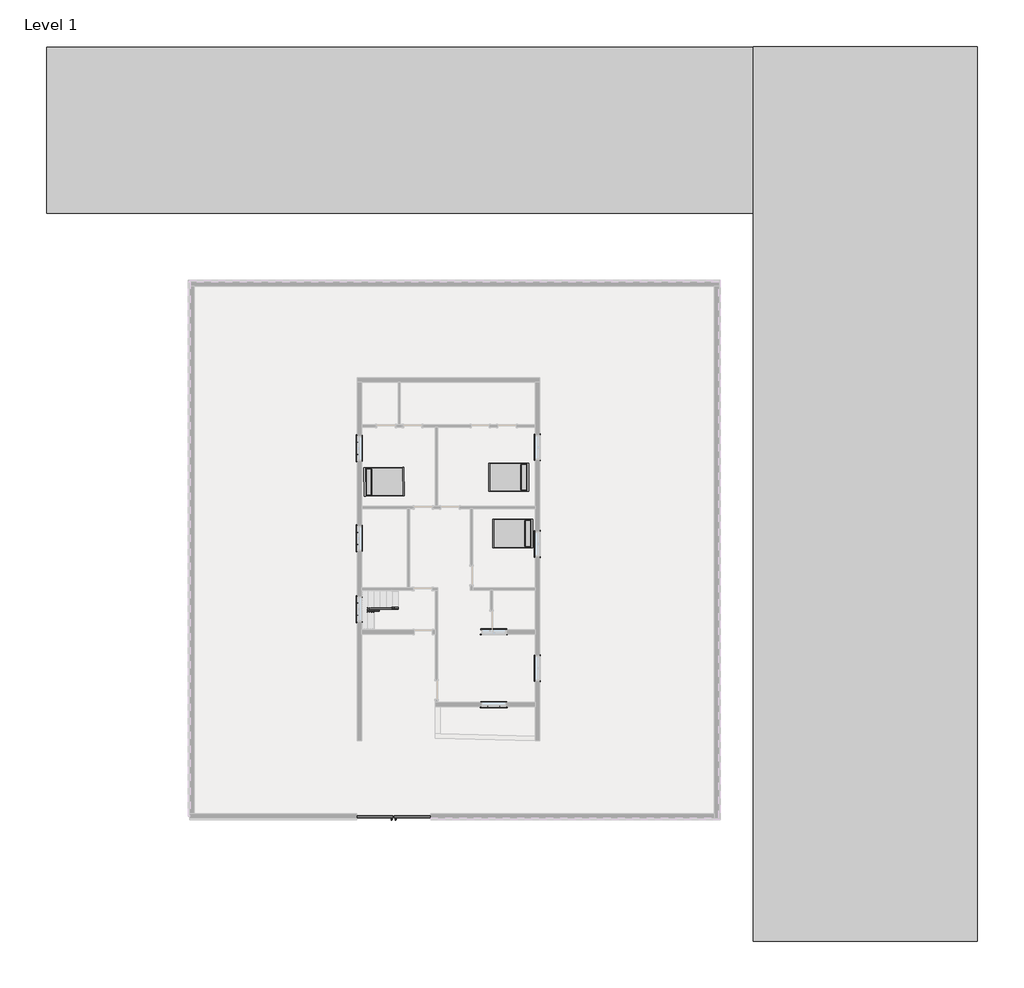
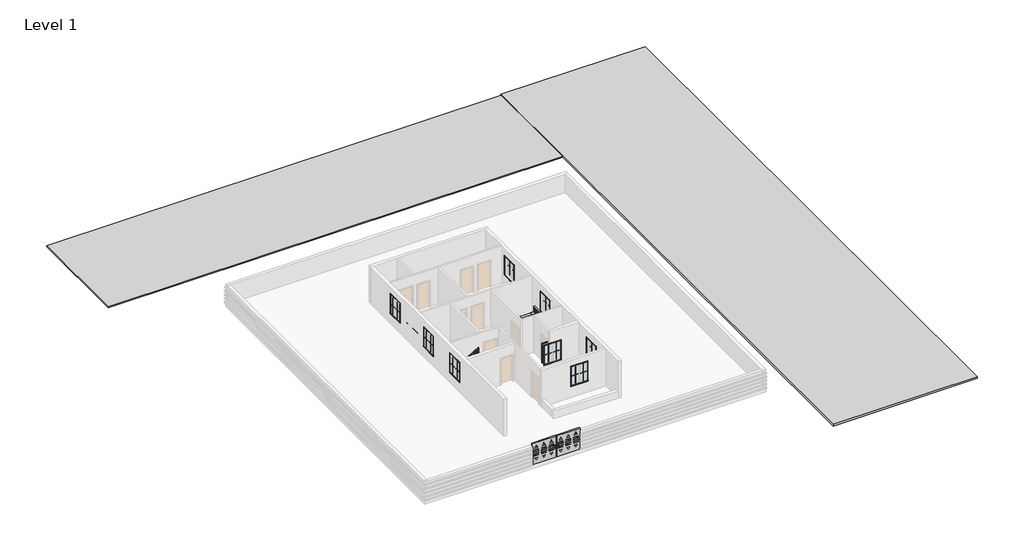
# One storey, part 3 of 3: 35 proxies, 3 furniture elements, 3 members, 1 railing.
"""IFC4 building model written with IfcOpenShell, lengths in millimetres."""

from ifc_helpers import new_model, si_unit, frame, origin, place, context, project, spatial, polyline, outline, extrude, faceted_brep, transform, mapped, element, save
from components import generic_models_af7f3ebe, generic_models_1_generic_models_1_dbe57743, generic_models_2_generic_models_2_6ec805a2, muntin_pattern_2x2_muntin_pattern_2x2_6dad3731, muntin_pattern_2x2_muntin_pattern_2x2_a30a3345, trim_window_exterior_flat_with_sill_92b9b949, trim_window_interior_flat_picture_frame_3bb882cf, furniture_121fd3aa

model = new_model("IFC4")

# Units and contexts
model_context = context("Model", 3, world=origin())
ifc_project = project(units=[si_unit("LENGTHUNIT", "METRE", prefix="MILLI")], contexts=[model_context])

# Site, building, storey
site = spatial("IfcSite", under=ifc_project)
building = spatial("IfcBuilding", under=site)
storey = spatial("IfcBuildingStorey", under=building, Name="Level 1", Elevation=0.0)

# Proxies
placement = place(None, origin())
generic_models_shape = generic_models_af7f3ebe(model_context)
element("IfcBuildingElementProxy", 1, Name="Generic Models", at=placement, inside=storey, context=model_context, shape_type="MappedRepresentation", body=[
    mapped(generic_models_shape, transform((2794.0, -7965.2365772, 0.0), x_axis=(1.0, 0.0, 0.0), y_axis=(0.0, 1.0, 0.0), z_axis=(0.0, 0.0, 1.0))),
])
generic_models_1_generic_models_1_shape = generic_models_1_generic_models_1_dbe57743(model_context)
element("IfcBuildingElementProxy", 2, Name="Generic Models 1 : Generic Models 1", ObjectType="Generic Models 1 : Generic Models 1", at=placement, inside=storey, context=model_context, shape_type="MappedRepresentation", body=[
    mapped(generic_models_1_generic_models_1_shape, transform((0.0, 0.0, 0.0), x_axis=(1.0, 0.0, 0.0), y_axis=(0.0, 1.0, 0.0), z_axis=(0.0, 0.0, 1.0))),
])
generic_models_2_generic_models_2_shape = generic_models_2_generic_models_2_6ec805a2(model_context)
element("IfcBuildingElementProxy", 3, Name="Generic Models 2 : Generic Models 2", ObjectType="Generic Models 2 : Generic Models 2", at=placement, inside=storey, context=model_context, shape_type="MappedRepresentation", body=[
    mapped(generic_models_2_generic_models_2_shape, transform((0.0, 0.0, 0.0), x_axis=(1.0, 0.0, 0.0), y_axis=(0.0, 1.0, 0.0), z_axis=(0.0, 0.0, 1.0))),
])
muntin_pattern_2x2_muntin_pattern_2x2_shape = muntin_pattern_2x2_muntin_pattern_2x2_6dad3731(model_context)
element("IfcBuildingElementProxy", 4, Name="Muntin Pattern_2x2 : Muntin Pattern_2x2", ObjectType="Muntin Pattern_2x2 : Muntin Pattern_2x2", at=placement, inside=storey, context=model_context, shape_type="MappedRepresentation", body=[
    mapped(muntin_pattern_2x2_muntin_pattern_2x2_shape, transform((1279.525, 5621.3375, 984.25), x_axis=(0.0, 1.0, 0.0), y_axis=(-1.0, 0.0, 0.0), z_axis=(0.0, 0.0, 1.0))),
])
element("IfcBuildingElementProxy", 5, Name="Muntin Pattern_2x2 : Muntin Pattern_2x2", ObjectType="Muntin Pattern_2x2 : Muntin Pattern_2x2", at=placement, inside=storey, context=model_context, shape_type="MappedRepresentation", body=[
    mapped(muntin_pattern_2x2_muntin_pattern_2x2_shape, transform((1279.525, 10129.8375, 984.25), x_axis=(0.0, 1.0, 0.0), y_axis=(-1.0, 0.0, 0.0), z_axis=(0.0, 0.0, 1.0))),
])
element("IfcBuildingElementProxy", 6, Name="Muntin Pattern_2x2 : Muntin Pattern_2x2", ObjectType="Muntin Pattern_2x2 : Muntin Pattern_2x2", at=placement, inside=storey, context=model_context, shape_type="MappedRepresentation", body=[
    mapped(muntin_pattern_2x2_muntin_pattern_2x2_shape, transform((10404.475, 10787.0625, 984.25), x_axis=(0.0, -1.0, 0.0), y_axis=(1.0, 0.0, 0.0), z_axis=(0.0, 0.0, 1.0))),
])
element("IfcBuildingElementProxy", 7, Name="Muntin Pattern_2x2 : Muntin Pattern_2x2", ObjectType="Muntin Pattern_2x2 : Muntin Pattern_2x2", at=placement, inside=storey, context=model_context, shape_type="MappedRepresentation", body=[
    mapped(muntin_pattern_2x2_muntin_pattern_2x2_shape, transform((10404.475, 5948.3625, 984.25), x_axis=(0.0, -1.0, 0.0), y_axis=(1.0, 0.0, 0.0), z_axis=(0.0, 0.0, 1.0))),
])
element("IfcBuildingElementProxy", 8, Name="Muntin Pattern_2x2 : Muntin Pattern_2x2", ObjectType="Muntin Pattern_2x2 : Muntin Pattern_2x2", at=placement, inside=storey, context=model_context, shape_type="MappedRepresentation", body=[
    mapped(muntin_pattern_2x2_muntin_pattern_2x2_shape, transform((10404.475, -274.6375, 984.25), x_axis=(0.0, -1.0, 0.0), y_axis=(1.0, 0.0, 0.0), z_axis=(0.0, 0.0, 1.0))),
])
element("IfcBuildingElementProxy", 9, Name="Muntin Pattern_2x2 : Muntin Pattern_2x2", ObjectType="Muntin Pattern_2x2 : Muntin Pattern_2x2", at=placement, inside=storey, context=model_context, shape_type="MappedRepresentation", body=[
    mapped(muntin_pattern_2x2_muntin_pattern_2x2_shape, transform((1279.525, 2078.0375, 984.25), x_axis=(0.0, 1.0, 0.0), y_axis=(-1.0, 0.0, 0.0), z_axis=(0.0, 0.0, 1.0))),
])
element("IfcBuildingElementProxy", 10, Name="Muntin Pattern_2x2 : Muntin Pattern_2x2", ObjectType="Muntin Pattern_2x2 : Muntin Pattern_2x2", at=placement, inside=storey, context=model_context, shape_type="MappedRepresentation", body=[
    mapped(muntin_pattern_2x2_muntin_pattern_2x2_shape, transform((8424.8625, 1139.825, 592.3065505), x_axis=(-1.0, 0.0, 0.0), y_axis=(0.0, -1.0, 0.0), z_axis=(0.0, 0.0, 1.0))),
])
element("IfcBuildingElementProxy", 11, Name="Muntin Pattern_2x2 : Muntin Pattern_2x2", ObjectType="Muntin Pattern_2x2 : Muntin Pattern_2x2", at=placement, inside=storey, context=model_context, shape_type="MappedRepresentation", body=[
    mapped(muntin_pattern_2x2_muntin_pattern_2x2_shape, transform((8418.5125, -2505.075, 1065.07095), x_axis=(-1.0, 0.0, 0.0), y_axis=(0.0, -1.0, 0.0), z_axis=(0.0, 0.0, 1.0))),
])
muntin_pattern_2x2_muntin_pattern_2x2_2_shape = muntin_pattern_2x2_muntin_pattern_2x2_a30a3345(model_context)
element("IfcBuildingElementProxy", 12, Name="Muntin Pattern_2x2 : Muntin Pattern_2x2", ObjectType="Muntin Pattern_2x2 : Muntin Pattern_2x2", at=placement, inside=storey, context=model_context, shape_type="MappedRepresentation", body=[
    mapped(muntin_pattern_2x2_muntin_pattern_2x2_2_shape, transform((1279.525, 6227.7625, 984.25), x_axis=(0.0, -1.0, 0.0), y_axis=(1.0, 0.0, 0.0), z_axis=(0.0, 0.0, 1.0))),
])
element("IfcBuildingElementProxy", 13, Name="Muntin Pattern_2x2 : Muntin Pattern_2x2", ObjectType="Muntin Pattern_2x2 : Muntin Pattern_2x2", at=placement, inside=storey, context=model_context, shape_type="MappedRepresentation", body=[
    mapped(muntin_pattern_2x2_muntin_pattern_2x2_2_shape, transform((1279.525, 10736.2625, 984.25), x_axis=(0.0, -1.0, 0.0), y_axis=(1.0, 0.0, 0.0), z_axis=(0.0, 0.0, 1.0))),
])
element("IfcBuildingElementProxy", 14, Name="Muntin Pattern_2x2 : Muntin Pattern_2x2", ObjectType="Muntin Pattern_2x2 : Muntin Pattern_2x2", at=placement, inside=storey, context=model_context, shape_type="MappedRepresentation", body=[
    mapped(muntin_pattern_2x2_muntin_pattern_2x2_2_shape, transform((10404.475, 10180.6375, 984.25), x_axis=(0.0, 1.0, 0.0), y_axis=(-1.0, 0.0, 0.0), z_axis=(0.0, 0.0, 1.0))),
])
element("IfcBuildingElementProxy", 15, Name="Muntin Pattern_2x2 : Muntin Pattern_2x2", ObjectType="Muntin Pattern_2x2 : Muntin Pattern_2x2", at=placement, inside=storey, context=model_context, shape_type="MappedRepresentation", body=[
    mapped(muntin_pattern_2x2_muntin_pattern_2x2_2_shape, transform((10404.475, 5341.9375, 984.25), x_axis=(0.0, 1.0, 0.0), y_axis=(-1.0, 0.0, 0.0), z_axis=(0.0, 0.0, 1.0))),
])
element("IfcBuildingElementProxy", 16, Name="Muntin Pattern_2x2 : Muntin Pattern_2x2", ObjectType="Muntin Pattern_2x2 : Muntin Pattern_2x2", at=placement, inside=storey, context=model_context, shape_type="MappedRepresentation", body=[
    mapped(muntin_pattern_2x2_muntin_pattern_2x2_2_shape, transform((10404.475, -881.0625, 984.25), x_axis=(0.0, 1.0, 0.0), y_axis=(-1.0, 0.0, 0.0), z_axis=(0.0, 0.0, 1.0))),
])
element("IfcBuildingElementProxy", 17, Name="Muntin Pattern_2x2 : Muntin Pattern_2x2", ObjectType="Muntin Pattern_2x2 : Muntin Pattern_2x2", at=placement, inside=storey, context=model_context, shape_type="MappedRepresentation", body=[
    mapped(muntin_pattern_2x2_muntin_pattern_2x2_2_shape, transform((1279.525, 2684.4625, 984.25), x_axis=(0.0, -1.0, 0.0), y_axis=(1.0, 0.0, 0.0), z_axis=(0.0, 0.0, 1.0))),
])
element("IfcBuildingElementProxy", 18, Name="Muntin Pattern_2x2 : Muntin Pattern_2x2", ObjectType="Muntin Pattern_2x2 : Muntin Pattern_2x2", at=placement, inside=storey, context=model_context, shape_type="MappedRepresentation", body=[
    mapped(muntin_pattern_2x2_muntin_pattern_2x2_2_shape, transform((7818.4375, 1139.825, 592.3065505), x_axis=(1.0, 0.0, 0.0), y_axis=(0.0, 1.0, 0.0), z_axis=(0.0, 0.0, 1.0))),
])
element("IfcBuildingElementProxy", 19, Name="Muntin Pattern_2x2 : Muntin Pattern_2x2", ObjectType="Muntin Pattern_2x2 : Muntin Pattern_2x2", at=placement, inside=storey, context=model_context, shape_type="MappedRepresentation", body=[
    mapped(muntin_pattern_2x2_muntin_pattern_2x2_2_shape, transform((7812.0875, -2505.075, 1065.07095), x_axis=(1.0, 0.0, 0.0), y_axis=(0.0, 1.0, 0.0), z_axis=(0.0, 0.0, 1.0))),
])
trim_window_exterior_flat_with_sill_shape = trim_window_exterior_flat_with_sill_92b9b949(model_context)
element("IfcBuildingElementProxy", 20, Name="Trim-Window-Exterior-Flat : with Sill", ObjectType="Trim-Window-Exterior-Flat : with Sill", at=placement, inside=storey, context=model_context, shape_type="MappedRepresentation", body=[
    mapped(trim_window_exterior_flat_with_sill_shape, transform((1270.0, 5924.55, 2438.4), x_axis=(0.0, -1.0, 0.0), y_axis=(0.0, 0.0, 1.0), z_axis=(-1.0, 0.0, 0.0))),
])
element("IfcBuildingElementProxy", 21, Name="Trim-Window-Exterior-Flat : with Sill", ObjectType="Trim-Window-Exterior-Flat : with Sill", at=placement, inside=storey, context=model_context, shape_type="MappedRepresentation", body=[
    mapped(trim_window_exterior_flat_with_sill_shape, transform((1270.0, 10433.05, 2438.4), x_axis=(0.0, -1.0, 0.0), y_axis=(0.0, 0.0, 1.0), z_axis=(-1.0, 0.0, 0.0))),
])
element("IfcBuildingElementProxy", 22, Name="Trim-Window-Exterior-Flat : with Sill", ObjectType="Trim-Window-Exterior-Flat : with Sill", at=placement, inside=storey, context=model_context, shape_type="MappedRepresentation", body=[
    mapped(trim_window_exterior_flat_with_sill_shape, transform((10414.0, 10483.85, 2438.4), x_axis=(0.0, 1.0, 0.0), y_axis=(0.0, 0.0, 1.0), z_axis=(1.0, 0.0, 0.0))),
])
element("IfcBuildingElementProxy", 23, Name="Trim-Window-Exterior-Flat : with Sill", ObjectType="Trim-Window-Exterior-Flat : with Sill", at=placement, inside=storey, context=model_context, shape_type="MappedRepresentation", body=[
    mapped(trim_window_exterior_flat_with_sill_shape, transform((10414.0, 5645.15, 2438.4), x_axis=(0.0, 1.0, 0.0), y_axis=(0.0, 0.0, 1.0), z_axis=(1.0, 0.0, 0.0))),
])
element("IfcBuildingElementProxy", 24, Name="Trim-Window-Exterior-Flat : with Sill", ObjectType="Trim-Window-Exterior-Flat : with Sill", at=placement, inside=storey, context=model_context, shape_type="MappedRepresentation", body=[
    mapped(trim_window_exterior_flat_with_sill_shape, transform((10414.0, -577.85, 2438.4), x_axis=(0.0, 1.0, 0.0), y_axis=(0.0, 0.0, 1.0), z_axis=(1.0, 0.0, 0.0))),
])
element("IfcBuildingElementProxy", 25, Name="Trim-Window-Exterior-Flat : with Sill", ObjectType="Trim-Window-Exterior-Flat : with Sill", at=placement, inside=storey, context=model_context, shape_type="MappedRepresentation", body=[
    mapped(trim_window_exterior_flat_with_sill_shape, transform((1270.0, 2381.25, 2438.4), x_axis=(0.0, -1.0, 0.0), y_axis=(0.0, 0.0, 1.0), z_axis=(-1.0, 0.0, 0.0))),
])
element("IfcBuildingElementProxy", 26, Name="Trim-Window-Exterior-Flat : with Sill", ObjectType="Trim-Window-Exterior-Flat : with Sill", at=placement, inside=storey, context=model_context, shape_type="MappedRepresentation", body=[
    mapped(trim_window_exterior_flat_with_sill_shape, transform((8121.65, 1130.3, 2046.4565505), x_axis=(1.0, 0.0, 0.0), y_axis=(0.0, 0.0, 1.0), z_axis=(0.0, -1.0, 0.0))),
])
element("IfcBuildingElementProxy", 27, Name="Trim-Window-Exterior-Flat : with Sill", ObjectType="Trim-Window-Exterior-Flat : with Sill", at=placement, inside=storey, context=model_context, shape_type="MappedRepresentation", body=[
    mapped(trim_window_exterior_flat_with_sill_shape, transform((8115.3, -2514.6, 2519.22095), x_axis=(1.0, 0.0, 0.0), y_axis=(0.0, 0.0, 1.0), z_axis=(0.0, -1.0, 0.0))),
])
trim_window_interior_flat_picture_frame_shape = trim_window_interior_flat_picture_frame_3bb882cf(model_context)
element("IfcBuildingElementProxy", 28, Name="Trim-Window-Interior-Flat : Picture Frame", ObjectType="Trim-Window-Interior-Flat : Picture Frame", at=placement, inside=storey, context=model_context, shape_type="MappedRepresentation", body=[
    mapped(trim_window_interior_flat_picture_frame_shape, transform((1498.6, 5924.55, 2438.4), x_axis=(0.0, 1.0, 0.0), y_axis=(0.0, 0.0, 1.0), z_axis=(1.0, 0.0, 0.0))),
])
element("IfcBuildingElementProxy", 29, Name="Trim-Window-Interior-Flat : Picture Frame", ObjectType="Trim-Window-Interior-Flat : Picture Frame", at=placement, inside=storey, context=model_context, shape_type="MappedRepresentation", body=[
    mapped(trim_window_interior_flat_picture_frame_shape, transform((1498.6, 10433.05, 2438.4), x_axis=(0.0, 1.0, 0.0), y_axis=(0.0, 0.0, 1.0), z_axis=(1.0, 0.0, 0.0))),
])
element("IfcBuildingElementProxy", 30, Name="Trim-Window-Interior-Flat : Picture Frame", ObjectType="Trim-Window-Interior-Flat : Picture Frame", at=placement, inside=storey, context=model_context, shape_type="MappedRepresentation", body=[
    mapped(trim_window_interior_flat_picture_frame_shape, transform((10185.4, 10483.85, 2438.4), x_axis=(0.0, -1.0, 0.0), y_axis=(0.0, 0.0, 1.0), z_axis=(-1.0, 0.0, 0.0))),
])
element("IfcBuildingElementProxy", 31, Name="Trim-Window-Interior-Flat : Picture Frame", ObjectType="Trim-Window-Interior-Flat : Picture Frame", at=placement, inside=storey, context=model_context, shape_type="MappedRepresentation", body=[
    mapped(trim_window_interior_flat_picture_frame_shape, transform((10185.4, 5645.15, 2438.4), x_axis=(0.0, -1.0, 0.0), y_axis=(0.0, 0.0, 1.0), z_axis=(-1.0, 0.0, 0.0))),
])
element("IfcBuildingElementProxy", 32, Name="Trim-Window-Interior-Flat : Picture Frame", ObjectType="Trim-Window-Interior-Flat : Picture Frame", at=placement, inside=storey, context=model_context, shape_type="MappedRepresentation", body=[
    mapped(trim_window_interior_flat_picture_frame_shape, transform((10185.4, -577.85, 2438.4), x_axis=(0.0, -1.0, 0.0), y_axis=(0.0, 0.0, 1.0), z_axis=(-1.0, 0.0, 0.0))),
])
element("IfcBuildingElementProxy", 33, Name="Trim-Window-Interior-Flat : Picture Frame", ObjectType="Trim-Window-Interior-Flat : Picture Frame", at=placement, inside=storey, context=model_context, shape_type="MappedRepresentation", body=[
    mapped(trim_window_interior_flat_picture_frame_shape, transform((1498.6, 2381.25, 2438.4), x_axis=(0.0, 1.0, 0.0), y_axis=(0.0, 0.0, 1.0), z_axis=(1.0, 0.0, 0.0))),
])
element("IfcBuildingElementProxy", 34, Name="Trim-Window-Interior-Flat : Picture Frame", ObjectType="Trim-Window-Interior-Flat : Picture Frame", at=placement, inside=storey, context=model_context, shape_type="MappedRepresentation", body=[
    mapped(trim_window_interior_flat_picture_frame_shape, transform((8121.65, 1358.9, 2046.4565505), x_axis=(-1.0, 0.0, 0.0), y_axis=(0.0, 0.0, 1.0), z_axis=(0.0, 1.0, 0.0))),
])
element("IfcBuildingElementProxy", 35, Name="Trim-Window-Interior-Flat : Picture Frame", ObjectType="Trim-Window-Interior-Flat : Picture Frame", at=placement, inside=storey, context=model_context, shape_type="MappedRepresentation", body=[
    mapped(trim_window_interior_flat_picture_frame_shape, transform((8115.3, -2286.0, 2519.22095), x_axis=(-1.0, 0.0, 0.0), y_axis=(0.0, 0.0, 1.0), z_axis=(0.0, 1.0, 0.0))),
])

# Furniture
furniture_shape = furniture_121fd3aa(model_context)
element("IfcFurniture", 36, ObjectType="Bed-Shaker : Double 56\" x 78\"", at=placement, inside=storey, context=model_context, shape_type="MappedRepresentation", body=[
    mapped(furniture_shape, transform((9849.8308516, 8970.3536289, 0.0), x_axis=(0.0, -1.0, 0.0), y_axis=(1.0, 0.0, 0.0), z_axis=(0.0, 0.0, 1.0))),
])
element("IfcFurniture", 37, ObjectType="Bed-Shaker : Double 56\" x 78\"", at=placement, inside=storey, context=model_context, shape_type="MappedRepresentation", body=[
    mapped(furniture_shape, transform((10050.5002502, 6155.12029, 0.0), x_axis=(0.0, -1.0, 0.0), y_axis=(1.0, 0.0, 0.0), z_axis=(0.0, 0.0, 1.0))),
])
element("IfcFurniture", 38, ObjectType="Bed-Shaker : Double 56\" x 78\"", at=placement, inside=storey, context=model_context, shape_type="MappedRepresentation", body=[
    mapped(furniture_shape, transform((1630.8006063, 8772.9712322, 0.0), x_axis=(-0.01124472055544287, 0.9999367761311863, 0.0), y_axis=(-0.9999367761311863, -0.01124472055544287, 0.0), z_axis=(0.0, 0.0, 1.0))),
])

# Members
element("IfcMember", 39, ObjectType="Stringer - 2\" Width", at=placement, inside=storey, context=model_context, shape_type="SweptSolid", body=[
    extrude(outline(polyline([(0.0, 3327.4), (207.5983948, 3327.4), (1026.0428392, 1854.2), (677.3641651, 1854.2), (0.0, 3073.4554972), (0.0, 3327.4)])), frame((0.0, 2374.9, 0.0), z_axis=(0.0, 1.0, 0.0), x_axis=(0.0, 0.0, 1.0)), (0.0, 0.0, 1.0), 50.8),
])
element("IfcMember", 40, ObjectType="Stringer - 2\" Width", at=placement, inside=storey, context=model_context, shape_type="SweptSolid", body=[
    extrude(outline(polyline([(1803.4, 2425.7), (1854.2, 2425.7), (1854.2, 2324.1), (1803.4, 2324.1), (1803.4, 2425.7)])), frame((0.0, 0.0, 787.4), z_axis=(0.0, 0.0, 1.0), x_axis=(1.0, 0.0, 0.0)), (0.0, 0.0, 1.0), 304.8),
])
element("IfcMember", 41, ObjectType="Stringer - 2\" Width", at=placement, inside=storey, context=model_context, shape_type="SweptSolid", body=[
    extrude(outline(polyline([(1223.5983948, 1803.4), (874.9197207, 1803.4), (1552.253054, 3022.6), (1900.9317281, 3022.6), (1223.5983948, 1803.4)])), frame((0.0, 2273.3, 0.0), z_axis=(0.0, 1.0, 0.0), x_axis=(0.0, 0.0, 1.0)), (0.0, 0.0, 1.0), 50.8),
])

# Railing
element("IfcRailing", 42, ObjectType="Handrail - Rectangular", at=placement, inside=storey, context=model_context, shape_type="SolidModel", body=[
    faceted_brep([(3327.4, 2425.7, 1083.7333333), (3327.4, 2425.7, 1025.620221), (3327.4, 2476.5, 1025.620221), (3327.4, 2476.5, 1083.7333333), (1879.6, 2425.7, 1888.0666667), (1828.8, 2425.7, 1858.1757765), (1828.8, 2476.5, 1858.1757765), (1879.6, 2476.5, 1888.0666667), (1879.6, 2425.7, 1930.4), (1828.8, 2425.7, 1879.6), (1828.8, 2476.5, 1879.6), (1879.6, 2476.5, 1930.4), (1803.4, 2425.7, 1930.4), (1803.4, 2425.7, 1879.6), (1752.6, 2476.5, 1879.6), (1752.6, 2476.5, 1930.4), (1803.4, 2349.5, 1930.4), (1803.4, 2298.7, 1879.6), (1752.6, 2298.7, 1879.6), (1752.6, 2349.5, 1930.4), (1803.4, 2349.5, 2142.0666667), (1803.4, 2298.7, 2091.2666667), (1752.6, 2298.7, 2091.2666667), (1752.6, 2349.5, 2142.0666667), (1803.4, 2273.3, 2142.0666667), (1803.4, 2273.3, 2091.2666667), (1752.6, 2222.5, 2091.2666667), (1752.6, 2222.5, 2142.0666667), (1879.6, 2273.3, 2142.0666667), (1892.7636022, 2273.3, 2091.2666667), (1892.7636022, 2222.5, 2091.2666667), (1879.6, 2222.5, 2142.0666667), (3022.6, 2273.3, 2777.0666667), (3022.6, 2222.5, 2777.0666667), (3022.6, 2222.5, 2718.9535543), (3022.6, 2273.3, 2718.9535543)], [[[0, 1, 2, 3]], [[1, 0, 4, 5]], [[2, 1, 5, 6]], [[3, 2, 6, 7]], [[0, 3, 7, 4]], [[5, 4, 8, 9]], [[6, 5, 9, 10]], [[7, 6, 10, 11]], [[4, 7, 11, 8]], [[9, 8, 12, 13]], [[10, 9, 13, 14]], [[11, 10, 14, 15]], [[8, 11, 15, 12]], [[13, 12, 16, 17]], [[14, 13, 17, 18]], [[15, 14, 18, 19]], [[12, 15, 19, 16]], [[17, 16, 20, 21]], [[18, 17, 21, 22]], [[19, 18, 22, 23]], [[16, 19, 23, 20]], [[21, 20, 24, 25]], [[22, 21, 25, 26]], [[23, 22, 26, 27]], [[20, 23, 27, 24]], [[25, 24, 28, 29]], [[26, 25, 29, 30]], [[27, 26, 30, 31]], [[24, 27, 31, 28]], [[32, 33, 34, 35]], [[29, 28, 32, 35]], [[30, 29, 35, 34]], [[31, 30, 34, 33]], [[28, 31, 33, 32]]]),
    extrude(outline(polyline([(2699.5507765, 2987.675), (1693.3333333, 2987.675), (1693.3333333, 3006.725), (2710.1341099, 3006.725), (2699.5507765, 2987.675)])), frame((0.0, 2238.375, 0.0), z_axis=(0.0, 1.0, 0.0), x_axis=(0.0, 0.0, 1.0)), (0.0, 0.0, 1.0), 19.05),
    extrude(outline(polyline([(2643.1063321, 2886.075), (1693.3333333, 2886.075), (1693.3333333, 2905.125), (2653.6896654, 2905.125), (2643.1063321, 2886.075)])), frame((0.0, 2238.375, 0.0), z_axis=(0.0, 1.0, 0.0), x_axis=(0.0, 0.0, 1.0)), (0.0, 0.0, 1.0), 19.05),
    extrude(outline(polyline([(2586.6618876, 2784.475), (1693.3333333, 2784.475), (1693.3333333, 2803.525), (2597.245221, 2803.525), (2586.6618876, 2784.475)])), frame((0.0, 2238.375, 0.0), z_axis=(0.0, 1.0, 0.0), x_axis=(0.0, 0.0, 1.0)), (0.0, 0.0, 1.0), 19.05),
    extrude(outline(polyline([(2530.2174432, 2682.875), (1524.0, 2682.875), (1524.0, 2701.925), (2540.8007765, 2701.925), (2530.2174432, 2682.875)])), frame((0.0, 2238.375, 0.0), z_axis=(0.0, 1.0, 0.0), x_axis=(0.0, 0.0, 1.0)), (0.0, 0.0, 1.0), 19.05),
    extrude(outline(polyline([(2473.7729988, 2581.275), (1524.0, 2581.275), (1524.0, 2600.325), (2484.3563321, 2600.325), (2473.7729988, 2581.275)])), frame((0.0, 2238.375, 0.0), z_axis=(0.0, 1.0, 0.0), x_axis=(0.0, 0.0, 1.0)), (0.0, 0.0, 1.0), 19.05),
    extrude(outline(polyline([(2417.3285543, 2479.675), (1524.0, 2479.675), (1524.0, 2498.725), (2427.9118876, 2498.725), (2417.3285543, 2479.675)])), frame((0.0, 2238.375, 0.0), z_axis=(0.0, 1.0, 0.0), x_axis=(0.0, 0.0, 1.0)), (0.0, 0.0, 1.0), 19.05),
    extrude(outline(polyline([(2360.8841099, 2378.075), (1354.6666667, 2378.075), (1354.6666667, 2397.125), (2371.4674432, 2397.125), (2360.8841099, 2378.075)])), frame((0.0, 2238.375, 0.0), z_axis=(0.0, 1.0, 0.0), x_axis=(0.0, 0.0, 1.0)), (0.0, 0.0, 1.0), 19.05),
    extrude(outline(polyline([(2304.4396654, 2276.475), (1354.6666667, 2276.475), (1354.6666667, 2295.525), (2315.0229988, 2295.525), (2304.4396654, 2276.475)])), frame((0.0, 2238.375, 0.0), z_axis=(0.0, 1.0, 0.0), x_axis=(0.0, 0.0, 1.0)), (0.0, 0.0, 1.0), 19.05),
    extrude(outline(polyline([(2247.995221, 2174.875), (1354.6666667, 2174.875), (1354.6666667, 2193.925), (2258.5785543, 2193.925), (2247.995221, 2174.875)])), frame((0.0, 2238.375, 0.0), z_axis=(0.0, 1.0, 0.0), x_axis=(0.0, 0.0, 1.0)), (0.0, 0.0, 1.0), 19.05),
    extrude(outline(polyline([(2191.5507765, 2073.275), (1185.3333333, 2073.275), (1185.3333333, 2092.325), (2202.1341099, 2092.325), (2191.5507765, 2073.275)])), frame((0.0, 2238.375, 0.0), z_axis=(0.0, 1.0, 0.0), x_axis=(0.0, 0.0, 1.0)), (0.0, 0.0, 1.0), 19.05),
    extrude(outline(polyline([(2135.1063321, 1971.675), (1185.3333333, 1971.675), (1185.3333333, 1990.725), (2145.6896654, 1990.725), (2135.1063321, 1971.675)])), frame((0.0, 2238.375, 0.0), z_axis=(0.0, 1.0, 0.0), x_axis=(0.0, 0.0, 1.0)), (0.0, 0.0, 1.0), 19.05),
    extrude(outline(polyline([(2078.6618876, 1870.075), (1185.3333333, 1870.075), (1185.3333333, 1889.125), (2089.245221, 1889.125), (2078.6618876, 1870.075)])), frame((0.0, 2238.375, 0.0), z_axis=(0.0, 1.0, 0.0), x_axis=(0.0, 0.0, 1.0)), (0.0, 0.0, 1.0), 19.05),
    extrude(outline(polyline([(1787.525, 2359.025), (1787.525, 2339.975), (1768.475, 2339.975), (1768.475, 2359.025), (1787.525, 2359.025)])), frame((0.0, 0.0, 1016.0), z_axis=(0.0, 0.0, 1.0), x_axis=(1.0, 0.0, 0.0)), (0.0, 0.0, 1.0), 863.6),
    extrude(outline(polyline([(1812.925, 2441.575), (1793.875, 2441.575), (1793.875, 2460.625), (1812.925, 2460.625), (1812.925, 2441.575)])), frame((0.0, 0.0, 1016.0), z_axis=(0.0, 0.0, 1.0), x_axis=(1.0, 0.0, 0.0)), (0.0, 0.0, 1.0), 863.6),
    extrude(outline(polyline([(1821.1341099, 1895.475), (846.6666667, 1895.475), (846.6666667, 1914.525), (1810.5507765, 1914.525), (1821.1341099, 1895.475)])), frame((0.0, 2441.575, 0.0), z_axis=(0.0, 1.0, 0.0), x_axis=(0.0, 0.0, 1.0)), (0.0, 0.0, 1.0), 19.05),
    extrude(outline(polyline([(1764.6896654, 1997.075), (846.6666667, 1997.075), (846.6666667, 2016.125), (1754.1063321, 2016.125), (1764.6896654, 1997.075)])), frame((0.0, 2441.575, 0.0), z_axis=(0.0, 1.0, 0.0), x_axis=(0.0, 0.0, 1.0)), (0.0, 0.0, 1.0), 19.05),
    extrude(outline(polyline([(1708.245221, 2098.675), (846.6666667, 2098.675), (846.6666667, 2117.725), (1697.6618876, 2117.725), (1708.245221, 2098.675)])), frame((0.0, 2441.575, 0.0), z_axis=(0.0, 1.0, 0.0), x_axis=(0.0, 0.0, 1.0)), (0.0, 0.0, 1.0), 19.05),
    extrude(outline(polyline([(1651.8007765, 2200.275), (677.3333333, 2200.275), (677.3333333, 2219.325), (1641.2174432, 2219.325), (1651.8007765, 2200.275)])), frame((0.0, 2441.575, 0.0), z_axis=(0.0, 1.0, 0.0), x_axis=(0.0, 0.0, 1.0)), (0.0, 0.0, 1.0), 19.05),
    extrude(outline(polyline([(1595.3563321, 2301.875), (677.3333333, 2301.875), (677.3333333, 2320.925), (1584.7729988, 2320.925), (1595.3563321, 2301.875)])), frame((0.0, 2441.575, 0.0), z_axis=(0.0, 1.0, 0.0), x_axis=(0.0, 0.0, 1.0)), (0.0, 0.0, 1.0), 19.05),
    extrude(outline(polyline([(1538.9118876, 2403.475), (677.3333333, 2403.475), (677.3333333, 2422.525), (1528.3285543, 2422.525), (1538.9118876, 2403.475)])), frame((0.0, 2441.575, 0.0), z_axis=(0.0, 1.0, 0.0), x_axis=(0.0, 0.0, 1.0)), (0.0, 0.0, 1.0), 19.05),
    extrude(outline(polyline([(1482.4674432, 2505.075), (508.0, 2505.075), (508.0, 2524.125), (1471.8841099, 2524.125), (1482.4674432, 2505.075)])), frame((0.0, 2441.575, 0.0), z_axis=(0.0, 1.0, 0.0), x_axis=(0.0, 0.0, 1.0)), (0.0, 0.0, 1.0), 19.05),
    extrude(outline(polyline([(1426.0229988, 2606.675), (508.0, 2606.675), (508.0, 2625.725), (1415.4396654, 2625.725), (1426.0229988, 2606.675)])), frame((0.0, 2441.575, 0.0), z_axis=(0.0, 1.0, 0.0), x_axis=(0.0, 0.0, 1.0)), (0.0, 0.0, 1.0), 19.05),
    extrude(outline(polyline([(1369.5785543, 2708.275), (508.0, 2708.275), (508.0, 2727.325), (1358.995221, 2727.325), (1369.5785543, 2708.275)])), frame((0.0, 2441.575, 0.0), z_axis=(0.0, 1.0, 0.0), x_axis=(0.0, 0.0, 1.0)), (0.0, 0.0, 1.0), 19.05),
    extrude(outline(polyline([(1313.1341099, 2809.875), (338.6666667, 2809.875), (338.6666667, 2828.925), (1302.5507765, 2828.925), (1313.1341099, 2809.875)])), frame((0.0, 2441.575, 0.0), z_axis=(0.0, 1.0, 0.0), x_axis=(0.0, 0.0, 1.0)), (0.0, 0.0, 1.0), 19.05),
    extrude(outline(polyline([(1256.6896654, 2911.475), (338.6666667, 2911.475), (338.6666667, 2930.525), (1246.1063321, 2930.525), (1256.6896654, 2911.475)])), frame((0.0, 2441.575, 0.0), z_axis=(0.0, 1.0, 0.0), x_axis=(0.0, 0.0, 1.0)), (0.0, 0.0, 1.0), 19.05),
    extrude(outline(polyline([(1200.245221, 3013.075), (338.6666667, 3013.075), (338.6666667, 3032.125), (1189.6618876, 3032.125), (1200.245221, 3013.075)])), frame((0.0, 2441.575, 0.0), z_axis=(0.0, 1.0, 0.0), x_axis=(0.0, 0.0, 1.0)), (0.0, 0.0, 1.0), 19.05),
    extrude(outline(polyline([(1143.8007765, 3114.675), (169.3333333, 3114.675), (169.3333333, 3133.725), (1133.2174432, 3133.725), (1143.8007765, 3114.675)])), frame((0.0, 2441.575, 0.0), z_axis=(0.0, 1.0, 0.0), x_axis=(0.0, 0.0, 1.0)), (0.0, 0.0, 1.0), 19.05),
    extrude(outline(polyline([(1087.3563321, 3216.275), (169.3333333, 3216.275), (169.3333333, 3235.325), (1076.7729988, 3235.325), (1087.3563321, 3216.275)])), frame((0.0, 2441.575, 0.0), z_axis=(0.0, 1.0, 0.0), x_axis=(0.0, 0.0, 1.0)), (0.0, 0.0, 1.0), 19.05),
    extrude(outline(polyline([(1787.525, 2257.425), (1787.525, 2238.375), (1768.475, 2238.375), (1768.475, 2257.425), (1787.525, 2257.425)])), frame((0.0, 0.0, 1016.0), z_axis=(0.0, 0.0, 1.0), x_axis=(1.0, 0.0, 0.0)), (0.0, 0.0, 1.0), 1075.2666667),
    extrude(outline(polyline([(1787.525, 2441.575), (1768.475, 2441.575), (1768.475, 2460.625), (1787.525, 2460.625), (1787.525, 2441.575)])), frame((0.0, 0.0, 1016.0), z_axis=(0.0, 0.0, 1.0), x_axis=(1.0, 0.0, 0.0)), (0.0, 0.0, 1.0), 863.6),
    extrude(outline(polyline([(2708.370221, 3003.55), (1693.3333333, 3003.55), (1693.3333333, 3022.6), (2718.9535543, 3022.6), (2708.370221, 3003.55)])), frame((0.0, 2238.375, 0.0), z_axis=(0.0, 1.0, 0.0), x_axis=(0.0, 0.0, 1.0)), (0.0, 0.0, 1.0), 19.05),
    extrude(outline(polyline([(1036.2035543, 3308.35), (169.3333333, 3308.35), (169.3333333, 3327.4), (1025.620221, 3327.4), (1036.2035543, 3308.35)])), frame((0.0, 2441.575, 0.0), z_axis=(0.0, 1.0, 0.0), x_axis=(0.0, 0.0, 1.0)), (0.0, 0.0, 1.0), 19.05),
])

save(model, "model.ifc")

# Revit data of these elements
# Type
#   Default Elevation = 0
# Type "Muntin Pattern_2x2 : Muntin Pattern_2x2"
#   Width [instance default] = 4' - 0"
#   Thickness = 0' - 0 1/2"
#   Height [instance default] = 4' - 0"
#   Distance = 0' - 0 3/4"
#   Interior Material [instance default] = none
#   Exterior Material [instance default] = none
#   Default Elevation = 0
# Type "Trim-Window-Exterior-Flat : with Sill"
#   Trim Width = 0' - 2 1/4"
#   Trim Thickness_Picture Frame = 0' - 1 1/4"
#   Trim Thickness_with Sill = 0' - 0 3/4"
#   Sill Thickness = 0' - 1 1/4"
#   Opening Width [instance default] = 2' - 0"
#   Opening Height [instance default] = 3' - 0"
#   Default Elevation = 4' - 0"
#   Sill = yes
#   Picture Frame = no
#   Trim Material [instance default] = none
# Type "Trim-Window-Interior-Flat : Picture Frame"
#   Trim Thickness_Picture Frame = 0' - 1 1/4"
#   Trim Width = 0' - 2 1/4"
#   Trim Thickness_with Sill = 0' - 0 3/4"
#   Sill Thickness = 0' - 1 1/4"
#   Opening Width [instance default] = 2' - 0"
#   Opening Height [instance default] = 3' - 0"
#   Default Elevation = 4' - 0"
#   Sill = no
#   Picture Frame = yes
#   Trim Material [instance default] = none
# Type "Bed-Shaker : Double 56\" x 78\""
#   Assembly Code = "E2020200"
#   Length = 6' - 6"
#   Width = 4' - 8"
#   Frame Material = Birch
#   Mattress Material = Linen, White
#   Default Elevation = 0
# Type "Handrail - Rectangular"
#   Assembly Code = "C2010400"
#   built-in parameter 1008612 = 0.0416667 (stored number, unit not read)
#   built-in parameter 1008611 = 0.0416667 (stored number, unit not read)
#   built-in parameter 1008609 = 0.333333 (stored number, unit not read)
#   built-in parameter 1008604 = 0.166667 (stored number, unit not read)
#   built-in parameter 1008603 = 0.166667 (stored number, unit not read)
#   Railing Height = 3' - 0"
#   built-in parameter 1008630 = 2
#   built-in parameter 1008610 = 2
#   built-in parameter 1008618 = Baluster - Square : 3/4"
# Element 1 (IfcBuildingElementProxy)
#   Phase Created = New Construction
#   Materials on its faces: "GATE"
# Element 2 (IfcBuildingElementProxy, "Generic Models 1 : Generic Models 1")
#   Phase Created = New Construction
# Element 3 (IfcBuildingElementProxy, "Generic Models 2 : Generic Models 2")
#   Phase Created = New Construction
# Elements 4, 5, 6, 7, 8, 9, 10, 11, 12, 13, 14, 15, 16, 17, 18, 19 (IfcBuildingElementProxy, "Muntin Pattern_2x2 : Muntin Pattern_2x2")
#   Width = 1' - 6 5/8"
#   Height = 4' - 6 1/2"
#   Interior Material = Wood - Stained
#   Exterior Material = Clad - White
#   Phase Created = New Construction
#   Materials on its faces: "Clad - White", "Wood - Stained"
# Elements 20, 21, 22, 23, 24, 25, 26, 27 (IfcBuildingElementProxy, "Trim-Window-Exterior-Flat : with Sill")
#   Opening Width = 4' - 0"
#   Opening Height = 5' - 0"
#   Trim Material = Clad - White
#   Phase Created = New Construction
#   Materials on its faces: "Clad - White"
# Elements 28, 29, 30, 31, 32, 33, 34, 35 (IfcBuildingElementProxy, "Trim-Window-Interior-Flat : Picture Frame")
#   Opening Width = 4' - 0"
#   Opening Height = 5' - 0"
#   Trim Material = Wood - Stained
#   Phase Created = New Construction
#   Materials on its faces: "Wood - Stained"
# Elements 36, 37, 38 (IfcFurniture, "Bed-Shaker : Double 56\" x 78\"")
#   Phase Created = New Construction
#   Materials on its faces: "Birch", "Linen, White"
# Elements 39, 40, 41 (IfcMember, "Stringer - 2\" Width")
#   Phase Created = New Construction
# Element 42 (IfcRailing, "Handrail - Rectangular")
#   Phase Created = New Construction
# Materials
#   "Birch": class "Wood", colour RGB 224 178 126, transparency 0, Description = "Betula Alleghaniensis", Cost = 0
#   "Linen, White": class "Textile", colour RGB 247 247 239, transparency 0, Description = "Linen, white", Cost = 0
#   "GATE": class "Generic", colour RGB 120 120 120, transparency 0, Cost = 0
#   "Clad - White": class "Wood", colour RGB 242 242 238, transparency 0, Cost = 0
#   "Wood - Stained": class "Wood", colour RGB 224 178 126, transparency 0, Cost = 0
